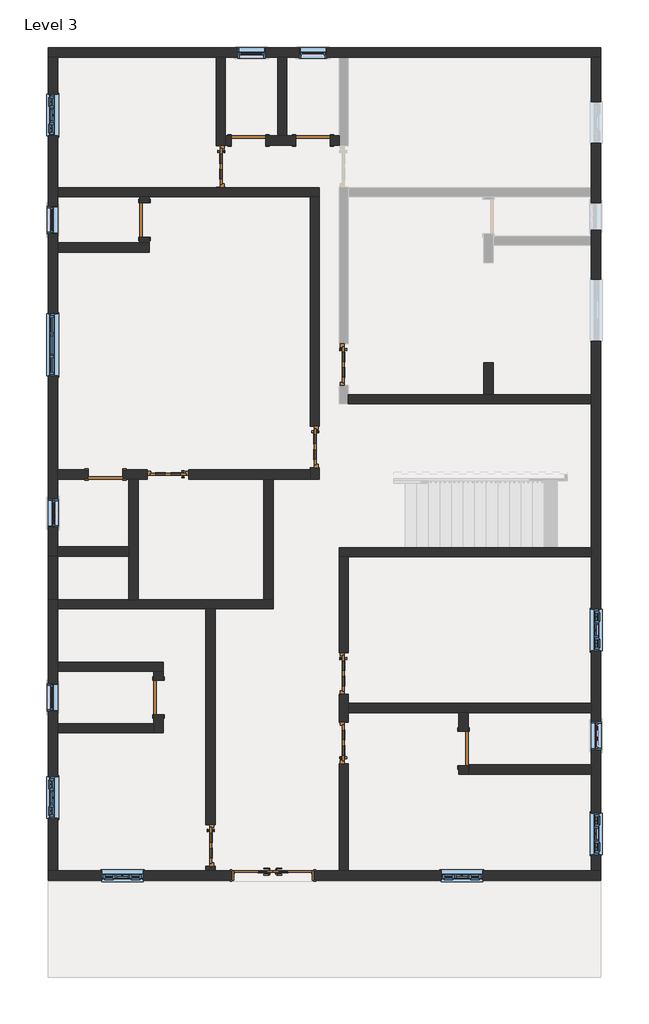
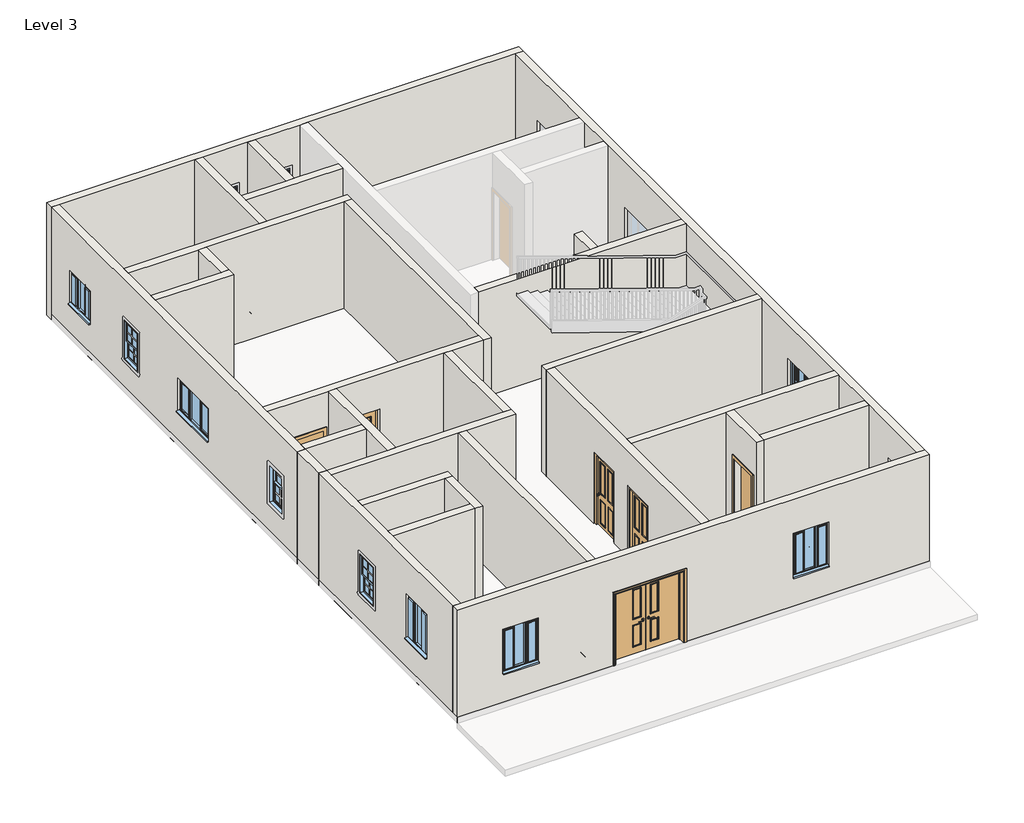
# One storey, part 1 of 3: 29 walls, 14 doors, 13 windows.
"""IFC4 building model written with IfcOpenShell, lengths in millimetres."""

from ifc_helpers import new_model, si_unit, frame, origin, place, context, project, spatial, polyline, outline, extrude, faceted_brep, transform, mapped, element, save
from components import door_2817e3e8, door_51b0c682, doors_intdbl_3_1810x2110mm_301b02ef, doors_intdbl_3_1810x2110mm_13513f6f, door_fadea3f2, door_53b1b562, window_679d2811, windows_tpl_plain_1360x910mm_84993ef1, windows_tpl_w_glazing_cross_bars_910x1210mm_e0b59135, windows_tpl_w_glazing_cross_bars_910x910mm_4aa0f884

model = new_model("IFC4")

# Units and contexts
model_context = context("Model", 3, world=origin())
ifc_project = project(units=[si_unit("LENGTHUNIT", "METRE", prefix="MILLI")], contexts=[model_context])

# Site, building, storey
site = spatial("IfcSite", under=ifc_project)
building = spatial("IfcBuilding", under=site)
storey = spatial("IfcBuildingStorey", under=building, Name="Level 3", Elevation=6096.0)

# Doors
placement = place(None, origin())
door_shape = door_2817e3e8(model_context)
element("IfcDoor", 1, ObjectType="Doors_ExtSgl_2 : 2'x7\"", at=placement, inside=storey, context=model_context, shape_type="MappedRepresentation", body=[
    mapped(door_shape, transform((-2349.4166288, 6357.8803322, 6096.0), x_axis=(0.0, -1.0, 0.0), y_axis=(1.0, 0.0, 0.0), z_axis=(0.0, 0.0, 1.0))),
])
element("IfcDoor", 2, ObjectType="Doors_ExtSgl_2 : 2'x7\"", at=placement, inside=storey, context=model_context, shape_type="MappedRepresentation", body=[
    mapped(door_shape, transform((-286.4451949, 208.0340986, 6096.0), x_axis=(0.0, -1.0, 0.0), y_axis=(1.0, 0.0, 0.0), z_axis=(0.0, 0.0, 1.0))),
])
element("IfcDoor", 3, ObjectType="Doors_ExtSgl_2 : 2'x7\"", at=placement, inside=storey, context=model_context, shape_type="MappedRepresentation", body=[
    mapped(door_shape, transform((348.5548051, -6285.6488489, 6096.0), x_axis=(0.0, 1.0, 0.0), y_axis=(-1.0, 0.0, 0.0), z_axis=(0.0, 0.0, 1.0))),
])
element("IfcDoor", 4, ObjectType="Doors_ExtSgl_2 : 2'x7\"", at=placement, inside=storey, context=model_context, shape_type="MappedRepresentation", body=[
    mapped(door_shape, transform((-2575.1220989, -8536.1734342, 6096.0), x_axis=(0.0, -1.0, 0.0), y_axis=(1.0, 0.0, 0.0), z_axis=(0.0, 0.0, 1.0))),
])
door_2_shape = door_51b0c682(model_context)
element("IfcDoor", 5, ObjectType="Doors_ExtSgl_2 : 2'x7\"", at=placement, inside=storey, context=model_context, shape_type="MappedRepresentation", body=[
    mapped(door_2_shape, transform((348.5548051, -4761.6488489, 6096.0), x_axis=(0.0, -1.0, 0.0), y_axis=(1.0, 0.0, 0.0), z_axis=(0.0, 0.0, 1.0))),
])
element("IfcDoor", 6, ObjectType="Doors_ExtSgl_2 : 2'x7\"", at=placement, inside=storey, context=model_context, shape_type="MappedRepresentation", body=[
    mapped(door_2_shape, transform((-3502.9153286, -401.5659014, 6096.0), x_axis=(-1.0, 0.0, 0.0), y_axis=(0.0, -1.0, 0.0), z_axis=(0.0, 0.0, 1.0))),
])
element("IfcDoor", 7, ObjectType="Doors_ExtSgl_2 : 2'x7\"", at=placement, inside=storey, context=model_context, shape_type="MappedRepresentation", body=[
    mapped(door_2_shape, transform((348.5548051, 2011.4340986, 6096.0), x_axis=(0.0, -1.0, 0.0), y_axis=(1.0, 0.0, 0.0), z_axis=(0.0, 0.0, 1.0))),
])
doors_intdbl_3_1810x2110mm_shape = doors_intdbl_3_1810x2110mm_301b02ef(model_context)
doors_intdbl_3_1810x2110mm_2_shape = doors_intdbl_3_1810x2110mm_13513f6f(model_context)
element("IfcDoor", 8, ObjectType="Doors_IntDbl_3 : 1810x2110mm", at=placement, inside=storey, context=model_context, shape_type="MappedRepresentation", body=[
    mapped(doors_intdbl_3_1810x2110mm_shape, transform((-1203.5220989, -9196.5734342, 6096.0), x_axis=(-1.0, 0.0, 0.0), y_axis=(0.0, -1.0, 0.0), z_axis=(0.0, 0.0, 1.0))),
    mapped(doors_intdbl_3_1810x2110mm_2_shape, transform((-1203.5220989, -9196.5734342, 6096.0), x_axis=(-1.0, 0.0, 0.0), y_axis=(0.0, -1.0, 0.0), z_axis=(0.0, 0.0, 1.0))),
])
door_3_shape = door_fadea3f2(model_context)
element("IfcDoor", 9, ObjectType="Single-Flush : 30\" x 80\"", at=placement, inside=storey, context=model_context, shape_type="MappedRepresentation", body=[
    mapped(door_3_shape, transform((-1739.8166288, 6926.3340986, 6096.0), x_axis=(1.0, 0.0, 0.0), y_axis=(0.0, 1.0, 0.0), z_axis=(0.0, 0.0, 1.0))),
])
element("IfcDoor", 10, ObjectType="Single-Flush : 30\" x 80\"", at=placement, inside=storey, context=model_context, shape_type="MappedRepresentation", body=[
    mapped(door_3_shape, transform((-4874.5153286, -401.5659014, 6096.0), x_axis=(-1.0, 0.0, 0.0), y_axis=(0.0, -1.0, 0.0), z_axis=(0.0, 0.0, 1.0))),
])
door_4_shape = door_53b1b562(model_context)
element("IfcDoor", 11, ObjectType="Single-Flush : 30\" x 80\"", at=placement, inside=storey, context=model_context, shape_type="MappedRepresentation", body=[
    mapped(door_4_shape, transform((-324.5451949, 6926.3340986, 6096.0), x_axis=(-1.0, 0.0, 0.0), y_axis=(0.0, -1.0, 0.0), z_axis=(0.0, 0.0, 1.0))),
])
element("IfcDoor", 12, ObjectType="Single-Flush : 30\" x 80\"", at=placement, inside=storey, context=model_context, shape_type="MappedRepresentation", body=[
    mapped(door_4_shape, transform((-3715.4451949, -5291.0659014, 6096.0), x_axis=(0.0, -1.0, 0.0), y_axis=(1.0, 0.0, 0.0), z_axis=(0.0, 0.0, 1.0))),
])
element("IfcDoor", 13, ObjectType="Single-Flush : 30\" x 80\"", at=placement, inside=storey, context=model_context, shape_type="MappedRepresentation", body=[
    mapped(door_4_shape, transform((2977.4548051, -6412.6488489, 6096.0), x_axis=(0.0, 1.0, 0.0), y_axis=(-1.0, 0.0, 0.0), z_axis=(0.0, 0.0, 1.0))),
])
element("IfcDoor", 14, ObjectType="Single-Flush : 30\" x 80\"", at=placement, inside=storey, context=model_context, shape_type="MappedRepresentation", body=[
    mapped(door_4_shape, transform((-4023.5839448, 5183.1303322, 6096.0), x_axis=(0.0, -1.0, 0.0), y_axis=(1.0, 0.0, 0.0), z_axis=(0.0, 0.0, 1.0))),
])

# Walls
element("IfcWall", 15, ObjectType="Generic - 4.5\" p", at=placement, inside=storey, context=model_context, shape_type="Brep", body=[
    faceted_brep([(-5928.5839448, 5687.8265658, 6096.0), (-4125.1839448, 5687.8265658, 6096.0), (-3921.9839448, 5687.8265658, 6096.0), (-388.0451949, 5687.8265658, 6096.0), (-184.8451949, 5687.8265658, 6096.0), (-184.8451949, 5687.8265658, 9144.0), (-388.0451949, 5687.8265658, 9144.0), (-3921.9839448, 5687.8265658, 9144.0), (-4125.1839448, 5687.8265658, 9144.0), (-5928.5839448, 5687.8265658, 9144.0), (-5928.5839448, 5891.0265658, 6096.0), (-5928.5839448, 5891.0265658, 9144.0), (-2451.0166288, 5891.0265658, 9144.0), (-2247.8166288, 5891.0265658, 9144.0), (-184.8451949, 5891.0265658, 9144.0), (-184.8451949, 5891.0265658, 6096.0), (-2247.8166288, 5891.0265658, 6096.0), (-2451.0166288, 5891.0265658, 6096.0)], [[[0, 1, 2, 3, 4, 5, 6, 7, 8, 9]], [[10, 11, 12, 13, 14, 15, 16, 17]], [[4, 3, 2, 1, 0, 10, 17, 16, 15]], [[0, 9, 11, 10]], [[5, 4, 15, 14]], [[9, 8, 7, 6, 5, 14, 13, 12, 11]]]),
])
element("IfcWall", 16, ObjectType="Generic - 4.5\" p", at=placement, inside=storey, context=model_context, shape_type="Brep", body=[
    faceted_brep([(-388.0451949, -246.9659014, 8206.0), (-388.0451949, -246.9659014, 6096.0), (-388.0451949, -299.9659014, 6096.0), (-388.0451949, -503.1659014, 6096.0), (-388.0451949, -503.1659014, 9144.0), (-388.0451949, -299.9659014, 9144.0), (-388.0451949, 5687.8265658, 9144.0), (-388.0451949, 5687.8265658, 6096.0), (-388.0451949, 663.0340986, 6096.0), (-388.0451949, 663.0340986, 8206.0), (-184.8451949, -503.1659014, 6096.0), (-184.8451949, -246.9659014, 6096.0), (-184.8451949, -246.9659014, 8206.0), (-184.8451949, 663.0340986, 8206.0), (-184.8451949, 663.0340986, 6096.0), (-184.8451949, 5687.8265658, 6096.0), (-184.8451949, 5687.8265658, 9144.0), (-184.8451949, -503.1659014, 9144.0)], [[[0, 1, 2, 3, 4, 5, 6, 7, 8, 9]], [[10, 11, 12, 13, 14, 15, 16, 17]], [[8, 7, 15, 14]], [[3, 2, 1, 11, 10]], [[7, 6, 16, 15]], [[4, 3, 10, 17]], [[14, 13, 9, 8]], [[12, 11, 1, 0]], [[13, 12, 0, 9]], [[6, 5, 4, 17, 16]]]),
])
element("IfcWall", 17, ObjectType="Generic - 4.5\" p", at=placement, inside=storey, context=model_context, shape_type="Brep", body=[
    faceted_brep([(-5255.5153286, -299.9659014, 8128.0), (-5255.5153286, -299.9659014, 6096.0), (-5928.5839448, -299.9659014, 6096.0), (-5928.5839448, -299.9659014, 9144.0), (-388.0451949, -299.9659014, 9144.0), (-388.0451949, -299.9659014, 6096.0), (-3047.9153286, -299.9659014, 6096.0), (-3047.9153286, -299.9659014, 8206.0), (-3957.9153286, -299.9659014, 8206.0), (-3957.9153286, -299.9659014, 6096.0), (-4493.5153286, -299.9659014, 6096.0), (-4493.5153286, -299.9659014, 8128.0), (-5928.5839448, -503.1659014, 6096.0), (-5255.5153286, -503.1659014, 6096.0), (-5255.5153286, -503.1659014, 8128.0), (-4493.5153286, -503.1659014, 8128.0), (-4493.5153286, -503.1659014, 6096.0), (-4366.5153286, -503.1659014, 6096.0), (-4163.3153286, -503.1659014, 6096.0), (-3957.9153286, -503.1659014, 6096.0), (-3957.9153286, -503.1659014, 8206.0), (-3047.9153286, -503.1659014, 8206.0), (-3047.9153286, -503.1659014, 6096.0), (-1404.0451949, -503.1659014, 6096.0), (-1200.8451949, -503.1659014, 6096.0), (-388.0451949, -503.1659014, 6096.0), (-388.0451949, -503.1659014, 9144.0), (-1200.8451949, -503.1659014, 9144.0), (-1404.0451949, -503.1659014, 9144.0), (-4163.3153286, -503.1659014, 9144.0), (-4366.5153286, -503.1659014, 9144.0), (-5928.5839448, -503.1659014, 9144.0)], [[[0, 1, 2, 3, 4, 5, 6, 7, 8, 9, 10, 11]], [[12, 13, 14, 15, 16, 17, 18, 19, 20, 21, 22, 23, 24, 25, 26, 27, 28, 29, 30, 31]], [[6, 5, 25, 24, 23, 22]], [[10, 9, 19, 18, 17, 16]], [[2, 1, 13, 12]], [[5, 4, 26, 25]], [[3, 2, 12, 31]], [[22, 21, 7, 6]], [[20, 19, 9, 8]], [[21, 20, 8, 7]], [[14, 13, 1, 0]], [[15, 14, 0, 11]], [[16, 15, 11, 10]], [[4, 3, 31, 30, 29, 28, 27, 26]]]),
])
element("IfcWall", 18, ObjectType="Generic - 4.5\" p", at=placement, inside=storey, context=model_context, shape_type="Brep", body=[
    faceted_brep([(-4366.5153286, -503.1659014, 6096.0), (-4366.5153286, -1989.0659014, 6096.0), (-4366.5153286, -2192.2659014, 6096.0), (-4366.5153286, -3144.7659014, 6096.0), (-4366.5153286, -3144.7659014, 9144.0), (-4366.5153286, -2192.2659014, 9144.0), (-4366.5153286, -1989.0659014, 9144.0), (-4366.5153286, -503.1659014, 9144.0), (-4163.3153286, -503.1659014, 6096.0), (-4163.3153286, -503.1659014, 9144.0), (-4163.3153286, -3144.7659014, 9144.0), (-4163.3153286, -3144.7659014, 6096.0)], [[[0, 1, 2, 3, 4, 5, 6, 7]], [[8, 9, 10, 11]], [[3, 2, 1, 0, 8, 11]], [[0, 7, 9, 8]], [[4, 3, 11, 10]], [[7, 6, 5, 4, 10, 9]]]),
])
element("IfcWall", 19, ObjectType="Generic - 4.5\" p", at=placement, inside=storey, context=model_context, shape_type="Brep", body=[
    faceted_brep([(-5928.5839448, -3347.9659014, 6096.0), (-2676.7220989, -3347.9659014, 6096.0), (-2473.5220989, -3347.9659014, 6096.0), (-1200.8451949, -3347.9659014, 6096.0), (-1200.8451949, -3347.9659014, 9144.0), (-2473.5220989, -3347.9659014, 9144.0), (-2676.7220989, -3347.9659014, 9144.0), (-5928.5839448, -3347.9659014, 9144.0), (-5928.5839448, -3144.7659014, 6096.0), (-5928.5839448, -3144.7659014, 9144.0), (-4366.5153286, -3144.7659014, 9144.0), (-4163.3153286, -3144.7659014, 9144.0), (-1404.0451949, -3144.7659014, 9144.0), (-1200.8451949, -3144.7659014, 9144.0), (-1200.8451949, -3144.7659014, 6096.0), (-1404.0451949, -3144.7659014, 6096.0), (-4163.3153286, -3144.7659014, 6096.0), (-4366.5153286, -3144.7659014, 6096.0)], [[[0, 1, 2, 3, 4, 5, 6, 7]], [[8, 9, 10, 11, 12, 13, 14, 15, 16, 17]], [[3, 2, 1, 0, 8, 17, 16, 15, 14]], [[0, 7, 9, 8]], [[4, 3, 14, 13]], [[7, 6, 5, 4, 13, 12, 11, 10, 9]]]),
])
element("IfcWall", 20, ObjectType="Generic - 4.5\" p", at=placement, inside=storey, context=model_context, shape_type="SweptSolid", body=[
    extrude(outline(polyline([(-4366.5153286, -2192.2659014), (-5928.5839448, -2192.2659014), (-5928.5839448, -1989.0659014), (-4366.5153286, -1989.0659014), (-4366.5153286, -2192.2659014)])), frame((0.0, 0.0, 6096.0), z_axis=(0.0, 0.0, 1.0), x_axis=(1.0, 0.0, 0.0)), (0.0, 0.0, 1.0), 3048.0),
])
element("IfcWall", 21, ObjectType="Generic - 4.5\" p", at=placement, inside=storey, context=model_context, shape_type="SweptSolid", body=[
    extrude(outline(polyline([(-1404.0451949, -3144.7659014), (-1404.0451949, -503.1659014), (-1200.8451949, -503.1659014), (-1200.8451949, -3144.7659014), (-1404.0451949, -3144.7659014)])), frame((0.0, 0.0, 6096.0), z_axis=(0.0, 0.0, 1.0), x_axis=(1.0, 0.0, 0.0)), (0.0, 0.0, 1.0), 3048.0),
])
element("IfcWall", 22, ObjectType="Generic - 4.5\" p", at=placement, inside=storey, context=model_context, shape_type="Brep", body=[
    faceted_brep([(-5928.5839448, -4719.5659014, 6096.0), (-3817.0451949, -4719.5659014, 6096.0), (-3613.8451949, -4719.5659014, 6096.0), (-3613.8451949, -4719.5659014, 9144.0), (-3817.0451949, -4719.5659014, 9144.0), (-5928.5839448, -4719.5659014, 9144.0), (-5928.5839448, -4516.3659014, 6096.0), (-5928.5839448, -4516.3659014, 9144.0), (-3613.8451949, -4516.3659014, 9144.0), (-3613.8451949, -4516.3659014, 6096.0)], [[[0, 1, 2, 3, 4, 5]], [[6, 7, 8, 9]], [[2, 1, 0, 6, 9]], [[0, 5, 7, 6]], [[3, 2, 9, 8]], [[5, 4, 3, 8, 7]]]),
])
element("IfcWall", 23, ObjectType="Generic - 4.5\" p", at=placement, inside=storey, context=model_context, shape_type="Brep", body=[
    faceted_brep([(-3817.0451949, -5672.0659014, 8128.0), (-3817.0451949, -5672.0659014, 6096.0), (-3817.0451949, -5862.5659014, 6096.0), (-3817.0451949, -6065.7659014, 6096.0), (-3817.0451949, -6065.7659014, 9144.0), (-3817.0451949, -5862.5659014, 9144.0), (-3817.0451949, -4719.5659014, 9144.0), (-3817.0451949, -4719.5659014, 6096.0), (-3817.0451949, -4910.0659014, 6096.0), (-3817.0451949, -4910.0659014, 8128.0), (-3613.8451949, -6065.7659014, 6096.0), (-3613.8451949, -5672.0659014, 6096.0), (-3613.8451949, -5672.0659014, 8128.0), (-3613.8451949, -4910.0659014, 8128.0), (-3613.8451949, -4910.0659014, 6096.0), (-3613.8451949, -4719.5659014, 6096.0), (-3613.8451949, -4719.5659014, 9144.0), (-3613.8451949, -6065.7659014, 9144.0)], [[[0, 1, 2, 3, 4, 5, 6, 7, 8, 9]], [[10, 11, 12, 13, 14, 15, 16, 17]], [[8, 7, 15, 14]], [[3, 2, 1, 11, 10]], [[7, 6, 16, 15]], [[4, 3, 10, 17]], [[12, 11, 1, 0]], [[13, 12, 0, 9]], [[14, 13, 9, 8]], [[6, 5, 4, 17, 16]]]),
])
element("IfcWall", 24, ObjectType="Generic - 4.5\" p", at=placement, inside=storey, context=model_context, shape_type="SweptSolid", body=[
    extrude(outline(polyline([(-5928.5839448, -5862.5659014), (-3817.0451949, -5862.5659014), (-3817.0451949, -6065.7659014), (-5928.5839448, -6065.7659014), (-5928.5839448, -5862.5659014)])), frame((0.0, 0.0, 6096.0), z_axis=(0.0, 0.0, 1.0), x_axis=(1.0, 0.0, 0.0)), (0.0, 0.0, 1.0), 3048.0),
])
element("IfcWall", 25, ObjectType="Generic - 4.5\" p", at=placement, inside=storey, context=model_context, shape_type="SweptSolid", body=[
    extrude(outline(polyline([(-8991.1734342, 8206.0), (-8991.1734342, 6096.0), (-9094.9734342, 6096.0), (-9094.9734342, 9144.0), (-3347.9659014, 9144.0), (-3347.9659014, 6096.0), (-8081.1734342, 6096.0), (-8081.1734342, 8206.0), (-8991.1734342, 8206.0)])), frame((-2676.7220989, 0.0, 0.0), z_axis=(1.0, 0.0, 0.0), x_axis=(0.0, 1.0, 0.0)), (0.0, 0.0, 1.0), 203.2),
])
element("IfcWall", 26, ObjectType="Generic - 4.5\" p", at=placement, inside=storey, context=model_context, shape_type="Brep", body=[
    faceted_brep([(-5928.5839448, 4475.2340986, 6096.0), (-3921.9839448, 4475.2340986, 6096.0), (-3921.9839448, 4475.2340986, 9144.0), (-5928.5839448, 4475.2340986, 9144.0), (-5928.5839448, 4678.4340986, 6096.0), (-5928.5839448, 4678.4340986, 9144.0), (-4125.1839448, 4678.4340986, 9144.0), (-3921.9839448, 4678.4340986, 9144.0), (-3921.9839448, 4678.4340986, 6096.0), (-4125.1839448, 4678.4340986, 6096.0)], [[[0, 1, 2, 3]], [[4, 5, 6, 7, 8, 9]], [[1, 0, 4, 9, 8]], [[0, 3, 5, 4]], [[2, 1, 8, 7]], [[3, 2, 7, 6, 5]]]),
])
element("IfcWall", 27, ObjectType="Generic - 4.5\" p", at=placement, inside=storey, context=model_context, shape_type="SweptSolid", body=[
    extrude(outline(polyline([(4802.1303322, 8128.0), (4802.1303322, 6096.0), (4678.4340986, 6096.0), (4678.4340986, 9144.0), (5687.8265658, 9144.0), (5687.8265658, 6096.0), (5564.1303322, 6096.0), (5564.1303322, 8128.0), (4802.1303322, 8128.0)])), frame((-4125.1839448, 0.0, 0.0), z_axis=(1.0, 0.0, 0.0), x_axis=(0.0, 1.0, 0.0)), (0.0, 0.0, 1.0), 203.2),
])
element("IfcWall", 28, ObjectType="Generic - 4.5\" p", at=placement, inside=storey, context=model_context, shape_type="Brep", body=[
    faceted_brep([(-2451.0166288, 5902.8803322, 8206.0), (-2451.0166288, 5902.8803322, 6096.0), (-2451.0166288, 5891.0265658, 6096.0), (-2451.0166288, 5891.0265658, 9144.0), (-2451.0166288, 8752.5974079, 9144.0), (-2451.0166288, 8752.5974079, 6096.0), (-2451.0166288, 6812.8803322, 6096.0), (-2451.0166288, 6812.8803322, 8206.0), (-2247.8166288, 5891.0265658, 6096.0), (-2247.8166288, 5902.8803322, 6096.0), (-2247.8166288, 5902.8803322, 8206.0), (-2247.8166288, 6812.8803322, 8206.0), (-2247.8166288, 6812.8803322, 6096.0), (-2247.8166288, 6824.7340986, 6096.0), (-2247.8166288, 7027.9340986, 6096.0), (-2247.8166288, 8752.5974079, 6096.0), (-2247.8166288, 8752.5974079, 9144.0), (-2247.8166288, 7027.9340986, 9144.0), (-2247.8166288, 6824.7340986, 9144.0), (-2247.8166288, 5891.0265658, 9144.0)], [[[0, 1, 2, 3, 4, 5, 6, 7]], [[8, 9, 10, 11, 12, 13, 14, 15, 16, 17, 18, 19]], [[6, 5, 15, 14, 13, 12]], [[2, 1, 9, 8]], [[5, 4, 16, 15]], [[3, 2, 8, 19]], [[12, 11, 7, 6]], [[10, 9, 1, 0]], [[11, 10, 0, 7]], [[4, 3, 19, 18, 17, 16]]]),
])
element("IfcWall", 29, ObjectType="Generic - 4.5\" p", at=placement, inside=storey, context=model_context, shape_type="Brep", body=[
    faceted_brep([(-1358.8166288, 6824.7340986, 6096.0), (-705.5451949, 6824.7340986, 6096.0), (-705.5451949, 6824.7340986, 8128.0), (56.4548051, 6824.7340986, 8128.0), (56.4548051, 6824.7340986, 6096.0), (246.9548051, 6824.7340986, 6096.0), (246.9548051, 6824.7340986, 9144.0), (-2247.8166288, 6824.7340986, 9144.0), (-2247.8166288, 6824.7340986, 6096.0), (-2120.8166288, 6824.7340986, 6096.0), (-2120.8166288, 6824.7340986, 8128.0), (-1358.8166288, 6824.7340986, 8128.0), (-705.5451949, 7027.9340986, 8128.0), (-705.5451949, 7027.9340986, 6096.0), (-896.0451949, 7027.9340986, 6096.0), (-1099.2451949, 7027.9340986, 6096.0), (-1358.8166288, 7027.9340986, 6096.0), (-1358.8166288, 7027.9340986, 8128.0), (-2120.8166288, 7027.9340986, 8128.0), (-2120.8166288, 7027.9340986, 6096.0), (-2247.8166288, 7027.9340986, 6096.0), (-2247.8166288, 7027.9340986, 9144.0), (-1099.2451949, 7027.9340986, 9144.0), (-896.0451949, 7027.9340986, 9144.0), (246.9548051, 7027.9340986, 9144.0), (246.9548051, 7027.9340986, 6096.0), (56.4548051, 7027.9340986, 6096.0), (56.4548051, 7027.9340986, 8128.0)], [[[0, 1, 2, 3, 4, 5, 6, 7, 8, 9, 10, 11]], [[12, 13, 14, 15, 16, 17, 18, 19, 20, 21, 22, 23, 24, 25, 26, 27]], [[9, 8, 20, 19]], [[26, 25, 5, 4]], [[16, 15, 14, 13, 1, 0]], [[8, 7, 21, 20]], [[6, 5, 25, 24]], [[17, 16, 0, 11]], [[18, 17, 11, 10]], [[19, 18, 10, 9]], [[2, 1, 13, 12]], [[3, 2, 12, 27]], [[4, 3, 27, 26]], [[7, 6, 24, 23, 22, 21]]]),
])
element("IfcWall", 30, ObjectType="Generic - 4.5\" p", at=placement, inside=storey, context=model_context, shape_type="SweptSolid", body=[
    extrude(outline(polyline([(-1099.2451949, 7027.9340986), (-1099.2451949, 8752.5974079), (-896.0451949, 8752.5974079), (-896.0451949, 7027.9340986), (-1099.2451949, 7027.9340986)])), frame((0.0, 0.0, 6096.0), z_axis=(0.0, 0.0, 1.0), x_axis=(1.0, 0.0, 0.0)), (0.0, 0.0, 1.0), 3048.0),
])
element("IfcWall", 31, ObjectType="Generic - 4.5\" p", at=placement, inside=storey, context=model_context, shape_type="Brep", body=[
    faceted_brep([(450.1548051, 1147.8340986, 6096.0), (5778.5439795, 1147.8340986, 6096.0), (5778.5439795, 1147.8340986, 9144.0), (450.1548051, 1147.8340986, 9144.0), (450.1548051, 1351.0340986, 6096.0), (450.1548051, 1351.0340986, 9144.0), (3421.9548051, 1351.0340986, 9144.0), (3625.1548051, 1351.0340986, 9144.0), (5778.5439795, 1351.0340986, 9144.0), (5778.5439795, 1351.0340986, 6096.0), (3625.1548051, 1351.0340986, 6096.0), (3421.9548051, 1351.0340986, 6096.0)], [[[0, 1, 2, 3]], [[4, 5, 6, 7, 8, 9, 10, 11]], [[1, 0, 4, 11, 10, 9]], [[0, 3, 5, 4]], [[2, 1, 9, 8]], [[3, 2, 8, 7, 6, 5]]]),
])
element("IfcWall", 32, ObjectType="Generic - 4.5\" p", at=placement, inside=storey, context=model_context, shape_type="SweptSolid", body=[
    extrude(outline(polyline([(3625.1548051, 2047.4361958), (3625.1548051, 1351.0340986), (3421.9548051, 1351.0340986), (3421.9548051, 2047.4361958), (3625.1548051, 2047.4361958)])), frame((0.0, 0.0, 6096.0), z_axis=(0.0, 0.0, 1.0), x_axis=(1.0, 0.0, 0.0)), (0.0, 0.0, 1.0), 3048.0),
])
element("IfcWall", 33, ObjectType="Generic - 4.5\" p", at=placement, inside=storey, context=model_context, shape_type="Brep", body=[
    faceted_brep([(5778.5439795, -2004.8977001, 6096.0), (246.9548051, -2004.8977001, 6096.0), (246.9548051, -2004.8977001, 9144.0), (5778.5439795, -2004.8977001, 9144.0), (5778.5439795, -2208.0977001, 6096.0), (5778.5439795, -2208.0977001, 9144.0), (450.1548051, -2208.0977001, 9144.0), (246.9548051, -2208.0977001, 9144.0), (246.9548051, -2208.0977001, 6096.0), (450.1548051, -2208.0977001, 6096.0)], [[[0, 1, 2, 3]], [[4, 5, 6, 7, 8, 9]], [[1, 0, 4, 9, 8]], [[0, 3, 5, 4]], [[2, 1, 8, 7]], [[3, 2, 7, 6, 5]]]),
])
element("IfcWall", 34, ObjectType="Generic - 4.5\" p", at=placement, inside=storey, context=model_context, shape_type="Brep", body=[
    faceted_brep([(246.9548051, -5216.6488489, 6096.0), (246.9548051, -5830.6488489, 6096.0), (246.9548051, -5830.6488489, 8206.0), (246.9548051, -6740.6488489, 8206.0), (246.9548051, -6740.6488489, 6096.0), (246.9548051, -9094.9734342, 6096.0), (246.9548051, -9094.9734342, 9144.0), (246.9548051, -2208.0977001, 9144.0), (246.9548051, -2208.0977001, 6096.0), (246.9548051, -4306.6488489, 6096.0), (246.9548051, -4306.6488489, 8206.0), (246.9548051, -5216.6488489, 8206.0), (450.1548051, -5830.6488489, 8206.0), (450.1548051, -5830.6488489, 6096.0), (450.1548051, -5625.2488489, 6096.0), (450.1548051, -5422.0488489, 6096.0), (450.1548051, -5216.6488489, 6096.0), (450.1548051, -5216.6488489, 8206.0), (450.1548051, -4306.6488489, 8206.0), (450.1548051, -4306.6488489, 6096.0), (450.1548051, -2208.0977001, 6096.0), (450.1548051, -2208.0977001, 9144.0), (450.1548051, -5422.0488489, 9144.0), (450.1548051, -5625.2488489, 9144.0), (450.1548051, -9094.9734342, 9144.0), (450.1548051, -9094.9734342, 6096.0), (450.1548051, -6740.6488489, 6096.0), (450.1548051, -6740.6488489, 8206.0)], [[[0, 1, 2, 3, 4, 5, 6, 7, 8, 9, 10, 11]], [[12, 13, 14, 15, 16, 17, 18, 19, 20, 21, 22, 23, 24, 25, 26, 27]], [[9, 8, 20, 19]], [[26, 25, 5, 4]], [[16, 15, 14, 13, 1, 0]], [[8, 7, 21, 20]], [[6, 5, 25, 24]], [[19, 18, 10, 9]], [[17, 16, 0, 11]], [[18, 17, 11, 10]], [[4, 3, 27, 26]], [[2, 1, 13, 12]], [[3, 2, 12, 27]], [[7, 6, 24, 23, 22, 21]]]),
])
element("IfcWall", 35, ObjectType="Generic - 4.5\" p", at=placement, inside=storey, context=model_context, shape_type="Brep", body=[
    faceted_brep([(450.1548051, -5625.2488489, 6096.0), (2875.8548051, -5625.2488489, 6096.0), (3079.0548051, -5625.2488489, 6096.0), (5778.5439795, -5625.2488489, 6096.0), (5778.5439795, -5625.2488489, 9144.0), (3079.0548051, -5625.2488489, 9144.0), (2875.8548051, -5625.2488489, 9144.0), (450.1548051, -5625.2488489, 9144.0), (450.1548051, -5422.0488489, 6096.0), (450.1548051, -5422.0488489, 9144.0), (5778.5439795, -5422.0488489, 9144.0), (5778.5439795, -5422.0488489, 6096.0)], [[[0, 1, 2, 3, 4, 5, 6, 7]], [[8, 9, 10, 11]], [[3, 2, 1, 0, 8, 11]], [[4, 3, 11, 10]], [[0, 7, 9, 8]], [[7, 6, 5, 4, 10, 9]]]),
])
element("IfcWall", 36, ObjectType="Generic - 4.5\" p", at=placement, inside=storey, context=model_context, shape_type="Brep", body=[
    faceted_brep([(2875.8548051, -5625.2488489, 6096.0), (2875.8548051, -6031.6488489, 6096.0), (2875.8548051, -6031.6488489, 8128.0), (2875.8548051, -6793.6488489, 8128.0), (2875.8548051, -6793.6488489, 6096.0), (2875.8548051, -6971.4488489, 6096.0), (2875.8548051, -6971.4488489, 9144.0), (2875.8548051, -5625.2488489, 9144.0), (3079.0548051, -6031.6488489, 8128.0), (3079.0548051, -6031.6488489, 6096.0), (3079.0548051, -5625.2488489, 6096.0), (3079.0548051, -5625.2488489, 9144.0), (3079.0548051, -6768.2488489, 9144.0), (3079.0548051, -6971.4488489, 9144.0), (3079.0548051, -6971.4488489, 6096.0), (3079.0548051, -6793.6488489, 6096.0), (3079.0548051, -6793.6488489, 8128.0)], [[[0, 1, 2, 3, 4, 5, 6, 7]], [[8, 9, 10, 11, 12, 13, 14, 15, 16]], [[10, 9, 1, 0]], [[15, 14, 5, 4]], [[0, 7, 11, 10]], [[6, 5, 14, 13]], [[2, 1, 9, 8]], [[3, 2, 8, 16]], [[4, 3, 16, 15]], [[7, 6, 13, 12, 11]]]),
])
element("IfcWall", 37, ObjectType="Generic - 4.5\" p", at=placement, inside=storey, context=model_context, shape_type="SweptSolid", body=[
    extrude(outline(polyline([(3079.0548051, -6768.2488489), (5778.5439795, -6768.2488489), (5778.5439795, -6971.4488489), (3079.0548051, -6971.4488489), (3079.0548051, -6768.2488489)])), frame((0.0, 0.0, 6096.0), z_axis=(0.0, 0.0, 1.0), x_axis=(1.0, 0.0, 0.0)), (0.0, 0.0, 1.0), 3048.0),
])
element("IfcWall", 38, ObjectType="Generic - 4.5\" p", at=placement, inside=storey, context=model_context, shape_type="SweptSolid", body=[
    extrude(outline(polyline([(-6131.7839448, -3144.7659014), (-6131.7839448, -2192.2659014), (-5928.5839448, -2192.2659014), (-5928.5839448, -3144.7659014), (-6131.7839448, -3144.7659014)])), frame((0.0, 0.0, 6096.0), z_axis=(0.0, 0.0, 1.0), x_axis=(1.0, 0.0, 0.0)), (0.0, 0.0, 1.0), 3048.0),
])
element("IfcWall", 39, ObjectType="Generic - 9\" w", at=placement, inside=storey, context=model_context, shape_type="Brep", body=[
    faceted_brep([(-6134.0560205, 8752.5974079, 6096.0), (-6131.7839448, 8752.5974079, 6096.0), (-5928.5839448, 8752.5974079, 6096.0), (-2451.0166288, 8752.5974079, 6096.0), (-2247.8166288, 8752.5974079, 6096.0), (-1099.2451949, 8752.5974079, 6096.0), (-896.0451949, 8752.5974079, 6096.0), (246.9548051, 8752.5974079, 6096.0), (450.1548051, 8752.5974079, 6096.0), (5778.5439795, 8752.5974079, 6096.0), (5981.7439795, 8752.5974079, 6096.0), (5981.7439795, 8752.5974079, 9144.0), (5778.5439795, 8752.5974079, 9144.0), (450.1548051, 8752.5974079, 9144.0), (246.9548051, 8752.5974079, 9144.0), (-896.0451949, 8752.5974079, 9144.0), (-1099.2451949, 8752.5974079, 9144.0), (-2247.8166288, 8752.5974079, 9144.0), (-2451.0166288, 8752.5974079, 9144.0), (-5928.5839448, 8752.5974079, 9144.0), (-6131.7839448, 8752.5974079, 9144.0), (-6134.0560205, 8752.5974079, 9144.0), (-1368.7309118, 8752.5974079, 8077.2), (-1368.7309118, 8752.5974079, 7010.4), (-1978.3309118, 8752.5974079, 7010.4), (-1978.3309118, 8752.5974079, 8077.2), (-19.7451949, 8752.5974079, 8077.2), (-19.7451949, 8752.5974079, 7010.4), (-629.3451949, 8752.5974079, 7010.4), (-629.3451949, 8752.5974079, 8077.2), (-6134.0560205, 8955.7974079, 6096.0), (-6134.0560205, 8955.7974079, 9144.0), (5981.7439795, 8955.7974079, 9144.0), (5981.7439795, 8955.7974079, 6096.0), (-1368.7309118, 8955.7974079, 8077.2), (-1978.3309118, 8955.7974079, 8077.2), (-1978.3309118, 8955.7974079, 7010.4), (-1368.7309118, 8955.7974079, 7010.4), (-19.7451949, 8955.7974079, 8077.2), (-629.3451949, 8955.7974079, 8077.2), (-629.3451949, 8955.7974079, 7010.4), (-19.7451949, 8955.7974079, 7010.4)], [[[0, 1, 2, 3, 4, 5, 6, 7, 8, 9, 10, 11, 12, 13, 14, 15, 16, 17, 18, 19, 20, 21], [22, 23, 24, 25], [26, 27, 28, 29]], [[30, 31, 32, 33], [34, 35, 36, 37], [38, 39, 40, 41]], [[10, 9, 8, 7, 6, 5, 4, 3, 2, 1, 0, 30, 33]], [[0, 21, 31, 30]], [[11, 10, 33, 32]], [[23, 22, 34, 37]], [[24, 23, 37, 36]], [[25, 24, 36, 35]], [[22, 25, 35, 34]], [[27, 26, 38, 41]], [[28, 27, 41, 40]], [[29, 28, 40, 39]], [[26, 29, 39, 38]], [[21, 20, 19, 18, 17, 16, 15, 14, 13, 12, 11, 32, 31]]]),
])
element("IfcWall", 40, ObjectType="Generic - 9\" w", at=placement, inside=storey, context=model_context, shape_type="Brep", body=[
    faceted_brep([(5981.7439795, -9094.9734342, 9144.0), (5981.7439795, -9094.9734342, 6096.0), (5778.5439795, -9094.9734342, 6096.0), (450.1548051, -9094.9734342, 6096.0), (246.9548051, -9094.9734342, 6096.0), (-298.5220989, -9094.9734342, 6096.0), (-298.5220989, -9094.9734342, 8206.0), (-2108.5220989, -9094.9734342, 8206.0), (-2108.5220989, -9094.9734342, 6096.0), (-2473.5220989, -9094.9734342, 6096.0), (-2676.7220989, -9094.9734342, 6096.0), (-5928.5839448, -9094.9734342, 6096.0), (-6131.7839448, -9094.9734342, 6096.0), (-6131.7839448, -9094.9734342, 9144.0), (-5928.5839448, -9094.9734342, 9144.0), (-2676.7220989, -9094.9734342, 9144.0), (-2473.5220989, -9094.9734342, 9144.0), (246.9548051, -9094.9734342, 9144.0), (450.1548051, -9094.9734342, 9144.0), (5778.5439795, -9094.9734342, 9144.0), (3394.3548051, -9094.9734342, 8220.4), (2484.3548051, -9094.9734342, 8220.4), (2484.3548051, -9094.9734342, 7010.4), (3394.3548051, -9094.9734342, 7010.4), (-4051.1839448, -9094.9734342, 8220.4), (-4961.1839448, -9094.9734342, 8220.4), (-4961.1839448, -9094.9734342, 7010.4), (-4051.1839448, -9094.9734342, 7010.4), (5981.7439795, -9298.1734342, 6096.0), (5981.7439795, -9298.1734342, 9144.0), (-6131.7839448, -9298.1734342, 9144.0), (-6131.7839448, -9298.1734342, 6096.0), (-2108.5220989, -9298.1734342, 6096.0), (-2108.5220989, -9298.1734342, 8206.0), (-298.5220989, -9298.1734342, 8206.0), (-298.5220989, -9298.1734342, 6096.0), (3394.3548051, -9298.1734342, 8220.4), (3394.3548051, -9298.1734342, 7010.4), (2484.3548051, -9298.1734342, 7010.4), (2484.3548051, -9298.1734342, 8220.4), (-4051.1839448, -9298.1734342, 8220.4), (-4051.1839448, -9298.1734342, 7010.4), (-4961.1839448, -9298.1734342, 7010.4), (-4961.1839448, -9298.1734342, 8220.4)], [[[0, 1, 2, 3, 4, 5, 6, 7, 8, 9, 10, 11, 12, 13, 14, 15, 16, 17, 18, 19], [20, 21, 22, 23], [24, 25, 26, 27]], [[28, 29, 30, 31, 32, 33, 34, 35], [36, 37, 38, 39], [40, 41, 42, 43]], [[1, 28, 35, 5, 4, 3, 2]], [[31, 12, 11, 10, 9, 8, 32]], [[1, 0, 29, 28]], [[13, 12, 31, 30]], [[7, 33, 32, 8]], [[33, 7, 6, 34]], [[34, 6, 5, 35]], [[37, 36, 20, 23]], [[38, 37, 23, 22]], [[39, 38, 22, 21]], [[36, 39, 21, 20]], [[41, 40, 24, 27]], [[42, 41, 27, 26]], [[43, 42, 26, 25]], [[40, 43, 25, 24]], [[0, 19, 18, 17, 16, 15, 14, 13, 30, 29]]]),
])
element("IfcWall", 41, ObjectType="Generic - 9\" w", at=placement, inside=storey, context=model_context, shape_type="Brep", body=[
    faceted_brep([(-5928.5839448, -9094.9734342, 6096.0), (-5928.5839448, -6065.7659014, 6096.0), (-5928.5839448, -5862.5659014, 6096.0), (-5928.5839448, -4719.5659014, 6096.0), (-5928.5839448, -4516.3659014, 6096.0), (-5928.5839448, -3347.9659014, 6096.0), (-5928.5839448, -3144.7659014, 6096.0), (-5928.5839448, -3144.7659014, 9144.0), (-5928.5839448, -3347.9659014, 9144.0), (-5928.5839448, -4516.3659014, 9144.0), (-5928.5839448, -4719.5659014, 9144.0), (-5928.5839448, -5862.5659014, 9144.0), (-5928.5839448, -6065.7659014, 9144.0), (-5928.5839448, -9094.9734342, 9144.0), (-5928.5839448, -7943.1659014, 8220.4), (-5928.5839448, -7033.1659014, 8220.4), (-5928.5839448, -7033.1659014, 7010.4), (-5928.5839448, -7943.1659014, 7010.4), (-5928.5839448, -5595.8659014, 8077.2), (-5928.5839448, -4986.2659014, 8077.2), (-5928.5839448, -4986.2659014, 7010.4), (-5928.5839448, -5595.8659014, 7010.4), (-6131.7839448, -9094.9734342, 6096.0), (-6131.7839448, -9094.9734342, 9144.0), (-6131.7839448, -3144.7659014, 9144.0), (-6131.7839448, -3144.7659014, 6096.0), (-6131.7839448, -7943.1659014, 8220.4), (-6131.7839448, -7943.1659014, 7010.4), (-6131.7839448, -7033.1659014, 7010.4), (-6131.7839448, -7033.1659014, 8220.4), (-6131.7839448, -5595.8659014, 8077.2), (-6131.7839448, -5595.8659014, 7010.4), (-6131.7839448, -4986.2659014, 7010.4), (-6131.7839448, -4986.2659014, 8077.2)], [[[0, 1, 2, 3, 4, 5, 6, 7, 8, 9, 10, 11, 12, 13], [14, 15, 16, 17], [18, 19, 20, 21]], [[22, 23, 24, 25], [26, 27, 28, 29], [30, 31, 32, 33]], [[6, 5, 4, 3, 2, 1, 0, 22, 25]], [[0, 13, 23, 22]], [[7, 6, 25, 24]], [[27, 26, 14, 17]], [[28, 27, 17, 16]], [[29, 28, 16, 15]], [[26, 29, 15, 14]], [[31, 30, 18, 21]], [[32, 31, 21, 20]], [[33, 32, 20, 19]], [[30, 33, 19, 18]], [[13, 12, 11, 10, 9, 8, 7, 24, 23]]]),
])
element("IfcWall", 42, ObjectType="Generic - 9\" w", at=placement, inside=storey, context=model_context, shape_type="Brep", body=[
    faceted_brep([(-5928.5839448, -2192.2659014, 6096.0), (-5928.5839448, -1989.0659014, 6096.0), (-5928.5839448, -503.1659014, 6096.0), (-5928.5839448, -299.9659014, 6096.0), (-5928.5839448, 4475.2340986, 6096.0), (-5928.5839448, 4678.4340986, 6096.0), (-5928.5839448, 5687.8265658, 6096.0), (-5928.5839448, 5891.0265658, 6096.0), (-5928.5839448, 8752.5974079, 6096.0), (-5928.5839448, 8752.5974079, 9144.0), (-5928.5839448, 5891.0265658, 9144.0), (-5928.5839448, 5687.8265658, 9144.0), (-5928.5839448, 4678.4340986, 9144.0), (-5928.5839448, 4475.2340986, 9144.0), (-5928.5839448, -299.9659014, 9144.0), (-5928.5839448, -503.1659014, 9144.0), (-5928.5839448, -1989.0659014, 9144.0), (-5928.5839448, -2192.2659014, 9144.0), (-5928.5839448, 1763.2340986, 7920.4), (-5928.5839448, 3123.2340986, 7920.4), (-5928.5839448, 3123.2340986, 7010.4), (-5928.5839448, 1763.2340986, 7010.4), (-5928.5839448, 7027.5974079, 7920.4), (-5928.5839448, 7937.5974079, 7920.4), (-5928.5839448, 7937.5974079, 7010.4), (-5928.5839448, 7027.5974079, 7010.4), (-5928.5839448, 4878.3303322, 8077.2), (-5928.5839448, 5487.9303322, 8077.2), (-5928.5839448, 5487.9303322, 7010.4), (-5928.5839448, 4878.3303322, 7010.4), (-5928.5839448, -941.3159014, 8077.2), (-5928.5839448, -941.3159014, 7010.4), (-5928.5839448, -1550.9159014, 7010.4), (-5928.5839448, -1550.9159014, 8077.2), (-6131.7839448, -2192.2659014, 6096.0), (-6131.7839448, -2192.2659014, 9144.0), (-6131.7839448, 8752.5974079, 9144.0), (-6131.7839448, 8752.5974079, 6096.0), (-6131.7839448, 1763.2340986, 7920.4), (-6131.7839448, 1763.2340986, 7010.4), (-6131.7839448, 3123.2340986, 7010.4), (-6131.7839448, 3123.2340986, 7920.4), (-6131.7839448, 7027.5974079, 7920.4), (-6131.7839448, 7027.5974079, 7010.4), (-6131.7839448, 7937.5974079, 7010.4), (-6131.7839448, 7937.5974079, 7920.4), (-6131.7839448, 4878.3303322, 8077.2), (-6131.7839448, 4878.3303322, 7010.4), (-6131.7839448, 5487.9303322, 7010.4), (-6131.7839448, 5487.9303322, 8077.2), (-6131.7839448, -941.3159014, 8077.2), (-6131.7839448, -1550.9159014, 8077.2), (-6131.7839448, -1550.9159014, 7010.4), (-6131.7839448, -941.3159014, 7010.4)], [[[0, 1, 2, 3, 4, 5, 6, 7, 8, 9, 10, 11, 12, 13, 14, 15, 16, 17], [18, 19, 20, 21], [22, 23, 24, 25], [26, 27, 28, 29], [30, 31, 32, 33]], [[34, 35, 36, 37], [38, 39, 40, 41], [42, 43, 44, 45], [46, 47, 48, 49], [50, 51, 52, 53]], [[8, 7, 6, 5, 4, 3, 2, 1, 0, 34, 37]], [[9, 8, 37, 36]], [[0, 17, 35, 34]], [[39, 38, 18, 21]], [[40, 39, 21, 20]], [[41, 40, 20, 19]], [[38, 41, 19, 18]], [[43, 42, 22, 25]], [[44, 43, 25, 24]], [[45, 44, 24, 23]], [[42, 45, 23, 22]], [[47, 46, 26, 29]], [[48, 47, 29, 28]], [[49, 48, 28, 27]], [[46, 49, 27, 26]], [[31, 30, 50, 53]], [[32, 31, 53, 52]], [[33, 32, 52, 51]], [[30, 33, 51, 50]], [[17, 16, 15, 14, 13, 12, 11, 10, 9, 36, 35]]]),
])
element("IfcWall", 43, ObjectType="Generic - 9\" w", at=placement, inside=storey, context=model_context, shape_type="Brep", body=[
    faceted_brep([(5778.5439795, 8752.5974079, 6096.0), (5778.5439795, 5891.0265658, 6096.0), (5778.5439795, 5687.8265658, 6096.0), (5778.5439795, 4830.8340986, 6096.0), (5778.5439795, 4627.6340986, 6096.0), (5778.5439795, 1351.0340986, 6096.0), (5778.5439795, 1147.8340986, 6096.0), (5778.5439795, -2004.8977001, 6096.0), (5778.5439795, -2208.0977001, 6096.0), (5778.5439795, -5422.0488489, 6096.0), (5778.5439795, -5625.2488489, 6096.0), (5778.5439795, -6768.2488489, 6096.0), (5778.5439795, -6971.4488489, 6096.0), (5778.5439795, -9094.9734342, 6096.0), (5778.5439795, -9094.9734342, 9144.0), (5778.5439795, -6971.4488489, 9144.0), (5778.5439795, -6768.2488489, 9144.0), (5778.5439795, -5625.2488489, 9144.0), (5778.5439795, -5422.0488489, 9144.0), (5778.5439795, -2208.0977001, 9144.0), (5778.5439795, -2004.8977001, 9144.0), (5778.5439795, 1147.8340986, 9144.0), (5778.5439795, 1351.0340986, 9144.0), (5778.5439795, 4627.6340986, 9144.0), (5778.5439795, 4830.8340986, 9144.0), (5778.5439795, 5687.8265658, 9144.0), (5778.5439795, 5891.0265658, 9144.0), (5778.5439795, 8752.5974079, 9144.0), (5778.5439795, -7827.1734342, 8220.4), (5778.5439795, -8737.1734342, 8220.4), (5778.5439795, -8737.1734342, 7010.4), (5778.5439795, -7827.1734342, 7010.4), (5778.5439795, -3360.0732745, 8220.4), (5778.5439795, -4270.0732745, 8220.4), (5778.5439795, -4270.0732745, 7010.4), (5778.5439795, -3360.0732745, 7010.4), (5778.5439795, 3885.2340986, 7920.4), (5778.5439795, 2525.2340986, 7920.4), (5778.5439795, 2525.2340986, 7010.4), (5778.5439795, 3885.2340986, 7010.4), (5778.5439795, 7776.8119869, 7920.4), (5778.5439795, 6866.8119869, 7920.4), (5778.5439795, 6866.8119869, 7010.4), (5778.5439795, 7776.8119869, 7010.4), (5778.5439795, 4954.5303322, 8077.2), (5778.5439795, 4954.5303322, 7010.4), (5778.5439795, 5564.1303322, 7010.4), (5778.5439795, 5564.1303322, 8077.2), (5778.5439795, -5828.4488489, 8077.2), (5778.5439795, -6438.0488489, 8077.2), (5778.5439795, -6438.0488489, 7010.4), (5778.5439795, -5828.4488489, 7010.4), (5981.7439795, 8752.5974079, 6096.0), (5981.7439795, 8752.5974079, 9144.0), (5981.7439795, -9094.9734342, 9144.0), (5981.7439795, -9094.9734342, 6096.0), (5981.7439795, -7827.1734342, 8220.4), (5981.7439795, -7827.1734342, 7010.4), (5981.7439795, -8737.1734342, 7010.4), (5981.7439795, -8737.1734342, 8220.4), (5981.7439795, -3360.0732745, 8220.4), (5981.7439795, -3360.0732745, 7010.4), (5981.7439795, -4270.0732745, 7010.4), (5981.7439795, -4270.0732745, 8220.4), (5981.7439795, 3885.2340986, 7920.4), (5981.7439795, 3885.2340986, 7010.4), (5981.7439795, 2525.2340986, 7010.4), (5981.7439795, 2525.2340986, 7920.4), (5981.7439795, 7776.8119869, 7920.4), (5981.7439795, 7776.8119869, 7010.4), (5981.7439795, 6866.8119869, 7010.4), (5981.7439795, 6866.8119869, 7920.4), (5981.7439795, 4954.5303322, 8077.2), (5981.7439795, 5564.1303322, 8077.2), (5981.7439795, 5564.1303322, 7010.4), (5981.7439795, 4954.5303322, 7010.4), (5981.7439795, -5828.4488489, 8077.2), (5981.7439795, -5828.4488489, 7010.4), (5981.7439795, -6438.0488489, 7010.4), (5981.7439795, -6438.0488489, 8077.2)], [[[0, 1, 2, 3, 4, 5, 6, 7, 8, 9, 10, 11, 12, 13, 14, 15, 16, 17, 18, 19, 20, 21, 22, 23, 24, 25, 26, 27], [28, 29, 30, 31], [32, 33, 34, 35], [36, 37, 38, 39], [40, 41, 42, 43], [44, 45, 46, 47], [48, 49, 50, 51]], [[52, 53, 54, 55], [56, 57, 58, 59], [60, 61, 62, 63], [64, 65, 66, 67], [68, 69, 70, 71], [72, 73, 74, 75], [76, 77, 78, 79]], [[13, 12, 11, 10, 9, 8, 7, 6, 5, 4, 3, 2, 1, 0, 52, 55]], [[0, 27, 53, 52]], [[14, 13, 55, 54]], [[57, 56, 28, 31]], [[58, 57, 31, 30]], [[59, 58, 30, 29]], [[56, 59, 29, 28]], [[61, 60, 32, 35]], [[62, 61, 35, 34]], [[63, 62, 34, 33]], [[60, 63, 33, 32]], [[65, 64, 36, 39]], [[66, 65, 39, 38]], [[67, 66, 38, 37]], [[64, 67, 37, 36]], [[69, 68, 40, 43]], [[70, 69, 43, 42]], [[71, 70, 42, 41]], [[68, 71, 41, 40]], [[45, 44, 72, 75]], [[46, 45, 75, 74]], [[47, 46, 74, 73]], [[44, 47, 73, 72]], [[77, 76, 48, 51]], [[78, 77, 51, 50]], [[79, 78, 50, 49]], [[76, 79, 49, 48]], [[27, 26, 25, 24, 23, 22, 21, 20, 19, 18, 17, 16, 15, 14, 54, 53]]]),
])

# Windows
window_shape = window_679d2811(model_context)
element("IfcWindow", 44, ObjectType="Window-Double-Hung : 24\" x 42\"", at=placement, inside=storey, context=model_context, shape_type="MappedRepresentation", body=[
    mapped(window_shape, transform((-6030.1839448, 5183.1303322, 6096.0), x_axis=(0.0, 1.0, 0.0), y_axis=(-1.0, 0.0, 0.0), z_axis=(0.0, 0.0, 1.0))),
])
element("IfcWindow", 45, ObjectType="Window-Double-Hung : 24\" x 42\"", at=placement, inside=storey, context=model_context, shape_type="MappedRepresentation", body=[
    mapped(window_shape, transform((-1673.5309118, 8854.1974079, 6096.0), x_axis=(-1.0, 0.0, 0.0), y_axis=(0.0, -1.0, 0.0), z_axis=(0.0, 0.0, 1.0))),
])
element("IfcWindow", 46, ObjectType="Window-Double-Hung : 24\" x 42\"", at=placement, inside=storey, context=model_context, shape_type="MappedRepresentation", body=[
    mapped(window_shape, transform((-324.5451949, 8854.1974079, 6096.0), x_axis=(-1.0, 0.0, 0.0), y_axis=(0.0, -1.0, 0.0), z_axis=(0.0, 0.0, 1.0))),
])
element("IfcWindow", 47, ObjectType="Window-Double-Hung : 24\" x 42\"", at=placement, inside=storey, context=model_context, shape_type="MappedRepresentation", body=[
    mapped(window_shape, transform((5880.1439795, -6133.2488489, 6096.0), x_axis=(0.0, -1.0, 0.0), y_axis=(1.0, 0.0, 0.0), z_axis=(0.0, 0.0, 1.0))),
])
element("IfcWindow", 48, ObjectType="Window-Double-Hung : 24\" x 42\"", at=placement, inside=storey, context=model_context, shape_type="MappedRepresentation", body=[
    mapped(window_shape, transform((-6030.1839448, -5291.0659014, 6096.0), x_axis=(0.0, 1.0, 0.0), y_axis=(-1.0, 0.0, 0.0), z_axis=(0.0, 0.0, 1.0))),
])
element("IfcWindow", 49, ObjectType="Window-Double-Hung : 24\" x 42\"", at=placement, inside=storey, context=model_context, shape_type="MappedRepresentation", body=[
    mapped(window_shape, transform((-6030.1839448, -1246.1159014, 6096.0), x_axis=(0.0, -1.0, 0.0), y_axis=(1.0, 0.0, 0.0), z_axis=(0.0, 0.0, 1.0))),
])
windows_tpl_plain_1360x910mm_shape = windows_tpl_plain_1360x910mm_84993ef1(model_context)
element("IfcWindow", 50, ObjectType="Windows_Tpl_Plain : 1360x910mm", at=placement, inside=storey, context=model_context, shape_type="MappedRepresentation", body=[
    mapped(windows_tpl_plain_1360x910mm_shape, transform((-6021.727377, 2944.9007653, 5810.4), x_axis=(0.0, 1.0, 0.0), y_axis=(-1.0, 0.0, 0.0), z_axis=(0.0, 0.0, 1.0))),
])
windows_tpl_w_glazing_cross_bars_910x1210mm_shape = windows_tpl_w_glazing_cross_bars_910x1210mm_e0b59135(model_context)
element("IfcWindow", 51, ObjectType="Windows_Tpl_w-Glazing_Cross-Bars : 910x1210mm", at=placement, inside=storey, context=model_context, shape_type="MappedRepresentation", body=[
    mapped(windows_tpl_w_glazing_cross_bars_910x1210mm_shape, transform((2512.6881384, -9188.1168663, 6110.4), x_axis=(-1.0, 0.0, 0.0), y_axis=(0.0, -1.0, 0.0), z_axis=(0.0, 0.0, 1.0))),
])
element("IfcWindow", 52, ObjectType="Windows_Tpl_w-Glazing_Cross-Bars : 910x1210mm", at=placement, inside=storey, context=model_context, shape_type="MappedRepresentation", body=[
    mapped(windows_tpl_w_glazing_cross_bars_910x1210mm_shape, transform((-4932.8506115, -9188.1168663, 6110.4), x_axis=(-1.0, 0.0, 0.0), y_axis=(0.0, -1.0, 0.0), z_axis=(0.0, 0.0, 1.0))),
])
element("IfcWindow", 53, ObjectType="Windows_Tpl_w-Glazing_Cross-Bars : 910x1210mm", at=placement, inside=storey, context=model_context, shape_type="MappedRepresentation", body=[
    mapped(windows_tpl_w_glazing_cross_bars_910x1210mm_shape, transform((-6021.727377, -7061.4992347, 6110.4), x_axis=(0.0, 1.0, 0.0), y_axis=(-1.0, 0.0, 0.0), z_axis=(0.0, 0.0, 1.0))),
])
element("IfcWindow", 54, ObjectType="Windows_Tpl_w-Glazing_Cross-Bars : 910x1210mm", at=placement, inside=storey, context=model_context, shape_type="MappedRepresentation", body=[
    mapped(windows_tpl_w_glazing_cross_bars_910x1210mm_shape, transform((5871.6874117, -8708.8401008, 6110.4), x_axis=(0.0, -1.0, 0.0), y_axis=(1.0, 0.0, 0.0), z_axis=(0.0, 0.0, 1.0))),
])
element("IfcWindow", 55, ObjectType="Windows_Tpl_w-Glazing_Cross-Bars : 910x1210mm", at=placement, inside=storey, context=model_context, shape_type="MappedRepresentation", body=[
    mapped(windows_tpl_w_glazing_cross_bars_910x1210mm_shape, transform((5871.6874117, -4241.7399412, 6110.4), x_axis=(0.0, -1.0, 0.0), y_axis=(1.0, 0.0, 0.0), z_axis=(0.0, 0.0, 1.0))),
])
windows_tpl_w_glazing_cross_bars_910x910mm_shape = windows_tpl_w_glazing_cross_bars_910x910mm_4aa0f884(model_context)
element("IfcWindow", 56, ObjectType="Windows_Tpl_w-Glazing_Cross-Bars : 910x910mm", at=placement, inside=storey, context=model_context, shape_type="MappedRepresentation", body=[
    mapped(windows_tpl_w_glazing_cross_bars_910x910mm_shape, transform((-6021.727377, 7909.2640745, 5810.4), x_axis=(0.0, 1.0, 0.0), y_axis=(-1.0, 0.0, 0.0), z_axis=(0.0, 0.0, 1.0))),
])

save(model, "model.ifc")

# Revit data of these elements
# Type "Doors_ExtSgl_2 : 2'x7\""
#   Type Mark = "10"
#   Type Comments = "External Single"
#   Operation = "SingleSwingRight"
#   Construction Type Id = "SGL"
#   Keynote = "L20"
#   Analytic Construction = "Large single-glazed windows"
#   Wrap Layers (Int) from Ext = 0' - 6.98819"
#   Wrap Layers (Ext) from Ext = 0' - 4.03543"
#   Visual Light Transmittance = 0.9
#   Thickness = 0' - 1.73228"
#   Stile Top of Lock rail = 3' - 3.37008"
#   Stile Top Rail = 0' - 5.90551"
#   Stile Shutting = 0' - 4.92126"
#   Stile Muntin Rail = 0' - 4.92126"
#   Stile Lock Rail = 0' - 6.88976"
#   Stile Hanging = 0' - 4.92126"
#   Stile Bottom Rail = 0' - 6.88976"
#   Solar Heat Gain Coefficient = 0.86
#   Rough Width = 2' - 11.82677"
#   Rough Height = 6' - 11.07087"
#   O/A Frame Width = 0' - 2.51969"
#   Heat Transfer Coefficient (U) = 0.979472 BTU/(h·ft²·°F)
#   Handle Z Distance = 3' - 3.37008"
#   Glazing Thickness = 0' - 0.94488"
#   FrameWidth = 0' - 1.65354"
#   FrameOffset - External = 0' - 0.98425"
#   FrameDepth = 0' - 3.50394"
#   Door Panel Width = 2' - 7.77165"
#   Door Panel Thickness = 0' - 1.73228"
#   Door Panel Height = 6' - 6.74016"
#   Cill Thickness = 0' - 2.14567"
#   Cill Projection = 0' - 1.1811"
#   Handle X Distance = 0' - 2.95276"
#   Height = 6' - 11.07087"
#   Structural Tolerance = 0' - 0.25591"
#   Tolerance = 0' - 0.11811"
#   Undercut = 0' - 0.15748"
#   Width = 2' - 11.82677"
#   Cill Extension = 0' - 0.98425"
#   Cavity Closer Width = 0' - 1.9685"
#   Cavity Closer Offset from Ext = 0' - 4.03543"
#   Cavity Closer Depth = 0' - 3.34646"
#   Vis - Ironmongery = yes
#   Vis - Cavity Closers = yes
#   Define Thermal Properties by = 1
#   Function = 1
#   Material Glass = Door - Glazing
#   Material Door = Door - Panel
#   Material Frame = Door - Frame/Mullion
#   Material Ironmongery = Door - Handle
#   Wall Closure = (empty or 0)
# Type "Doors_IntDbl_3 : 1810x2110mm"
#   Type Mark = "11"
#   Type Comments = "Internal Double"
#   Operation = "DoubleDoorSingleSwing"
#   Construction Type Id = "GSP4R"
#   Keynote = "L20"
#   Description = "Internal Double Door"
#   Analytic Construction = "1/8 in Pilkington single glazing"
#   Visual Light Transmittance = 0.9
#   VisionPanel Width = 0' - 7.87402"
#   Thickness = 0' - 1.25984"
#   Stop Thickness = 0' - 0.74803"
#   Stop Depth = 0' - 1.25984"
#   Stile Top Rail = 0' - 8.85827"
#   Stile Shutting = 0' - 4.92126"
#   Stile Lock Rail = 0' - 6.88976"
#   Stile Top of Lock Rail = 3' - 7.30709"
#   Stile Bottom Rail = 1' - 1.77953"
#   Solar Heat Gain Coefficient = 0.78
#   Rough Width = 5' - 11.25984"
#   Rough Height = 6' - 11.07087"
#   Heat Transfer Coefficient (U) = 0.6496 BTU/(h·ft²·°F)
#   Handle Z Distance = 3' - 3.37008"
#   Handle X Distance = 0' - 2.95276"
#   Frame Thickness = 0' - 1.25984"
#   Door Panel Width = 2' - 9.87795"
#   Door Panel Thickness = 0' - 1.25984"
#   Door Panel Height = 6' - 9.10236"
#   Height = 6' - 11.07087"
#   Door Panel Offset = 0' - 0"
#   Structural Tolerance = 0' - 0.31496"
#   Tolerance = 0' - 0.11811"
#   UnderCut = 0' - 0.27559"
#   Width = 5' - 11.25984"
#   Architrave Setback = 0' - 0.19685"
#   Vis - Ironmongery = yes
#   Define Thermal Properties by = 1
#   Material Ironmongery = Door - Handle
#   Material Glass = Door - Glazing
#   Material Frame = Door - Frame/Mullion
#   Material Door = Door - Panel
#   Material Beading = Door - Panel
#   Material Architrave = Door - Architrave
#   Function = (empty or 0)
#   Wall Closure = (empty or 0)
# Type "Single-Flush : 30\" x 80\""
#   Type Mark = "5"
#   Construction Type Id = "MDOOR"
#   Assembly Code = "C1020"
#   Analytic Construction = "Metal"
#   Thickness = 0' - 2"
#   Heat Transfer Coefficient (U) = 0.651978 BTU/(h·ft²·°F)
#   Height = 6' - 8"
#   Trim Projection Ext = 0' - 1"
#   Trim Projection Int = 0' - 1"
#   Trim Width = 0' - 3"
#   Width = 2' - 6"
#   Define Thermal Properties by = 1
#   Define Thermal Properties by = 1
#   Door Material = Door - Panel
#   Frame Material = Door - Frame
#   Visual Light Transmittance = 0
#   Solar Heat Gain Coefficient = 0
#   Function = (empty or 0)
#   Wall Closure = (empty or 0)
# Type "Generic - 4.5\" p"
#   Assembly Code = "B2010"
#   Layers, outside or top first: 0' - 8" no material (function 1)
# Type "Generic - 9\" w"
#   Assembly Code = "B2010"
#   Layers, outside or top first: 0' - 8" no material (function 1)
# Type "Window-Double-Hung : 24\" x 42\""
#   Type Mark = "10"
#   Fire Rating = "0.5h"
#   Construction Type Id = "DG-DR"
#   Assembly Code = "B2020100"
#   Analytic Construction = "Double glazing - domestic"
#   Wall Thickness [instance default] = 0' - 6"
#   Window Inset [instance default] = 0' - 0"
#   Visual Light Transmittance = 0.81
#   Thermal Resistance (R) = 1.8146 (h·ft²·°F)/BTU
#   Solar Heat Gain Coefficient = 0.76
#   Muntin Width = 1' - 6"
#   Muntin Height = 1' - 5 1/8"
#   Interior Wall Closure [instance default] = 0' - 1 1/2"
#   Rough Width = 2' - 0 1/2"
#   Rough Height = 3' - 6 1/2"
#   Frame Extension [instance default] = 0' - 1 1/4"
#   Exterior Wall Closure [instance default] = 0' - 0 1/2"
#   Extension Jamb [instance default] = 0' - 1 1/2"
#   Heat Transfer Coefficient (U) = 0.5511 BTU/(h·ft²·°F)
#   Height = 3' - 6"
#   Width = 2' - 0"
#   Define Thermal Properties by = 1
#   Top Muntin Visibility = yes
#   Indicator Visibility [instance default] = yes
#   Extension Jamb Visibility [instance default] = yes
#   Interior Trim Visibility [instance default] = yes
#   Exterior Trim Visibility [instance default] = yes
#   Define Thermal Properties by = 1
#   Bottom Muntin Visibility = yes
#   Muntin Pattern = Muntin Pattern_2x2 : Muntin Pattern_2x2
#   Interior Trim Material = Wood - Stained
#   Interior Trim = Trim-Window-Interior-Flat : Picture Frame
#   Exterior Trim Material = Clad - White
#   Exterior Trim = Trim-Window-Exterior-Flat : with Sill
#   Glass Panel Material = Glass
#   Exterior Frame Material = Clad - White
#   Interior Frame Material = Wood - Stained
#   Wall Closure = (empty or 0)
# Type "Windows_Tpl_Plain : 1360x910mm"
#   Type Mark = "20"
#   Operation = "TriplePanelVertical"
#   Construction Type Id = "GSP4R"
#   Manufacturer = "Revit"
#   Keynote = "L10"
#   Analytic Construction = "1/8 in Pilkington single glazing"
#   Wrap Layers (Ext) from Ext = 0' - 4.03543"
#   Wrap Layers (Int) from Ext = 0' - 6.98819"
#   Window Board Projection = 0' - 0.98425"
#   Window Board Extension = 0' - 0.98425"
#   Visual Light Transmittance = 0.9
#   Solar Heat Gain Coefficient = 0.78
#   Rough Width = 4' - 5.54331"
#   Rough Height = 2' - 11.82677"
#   Height = 2' - 11.82677"
#   Width = 4' - 5.54331"
#   Heat Transfer Coefficient (U) = 0.6496 BTU/(h·ft²·°F)
#   Glazing Thickness = 0' - 0.94488"
#   FrameOffset - External = 0' - 1.9685"
#   Frame Depth = 0' - 2.55906"
#   Default Head Height = 6' - 11.07087"
#   Cill Depth = 0' - 3.44488"
#   Cavity Closer Width = 0' - 1.9685"
#   Cavity Closer Offset from Ext = 0' - 4.03543"
#   Cavity Closer Depth = 0' - 3.34646"
#   Vis - Cavity Closers = yes
#   Define Thermal Properties by = 1
#   Material Trim = Window Frame
#   Material Glass = Glass
#   Material Frame = Window Frame
#   Wall Closure = (empty or 0)
